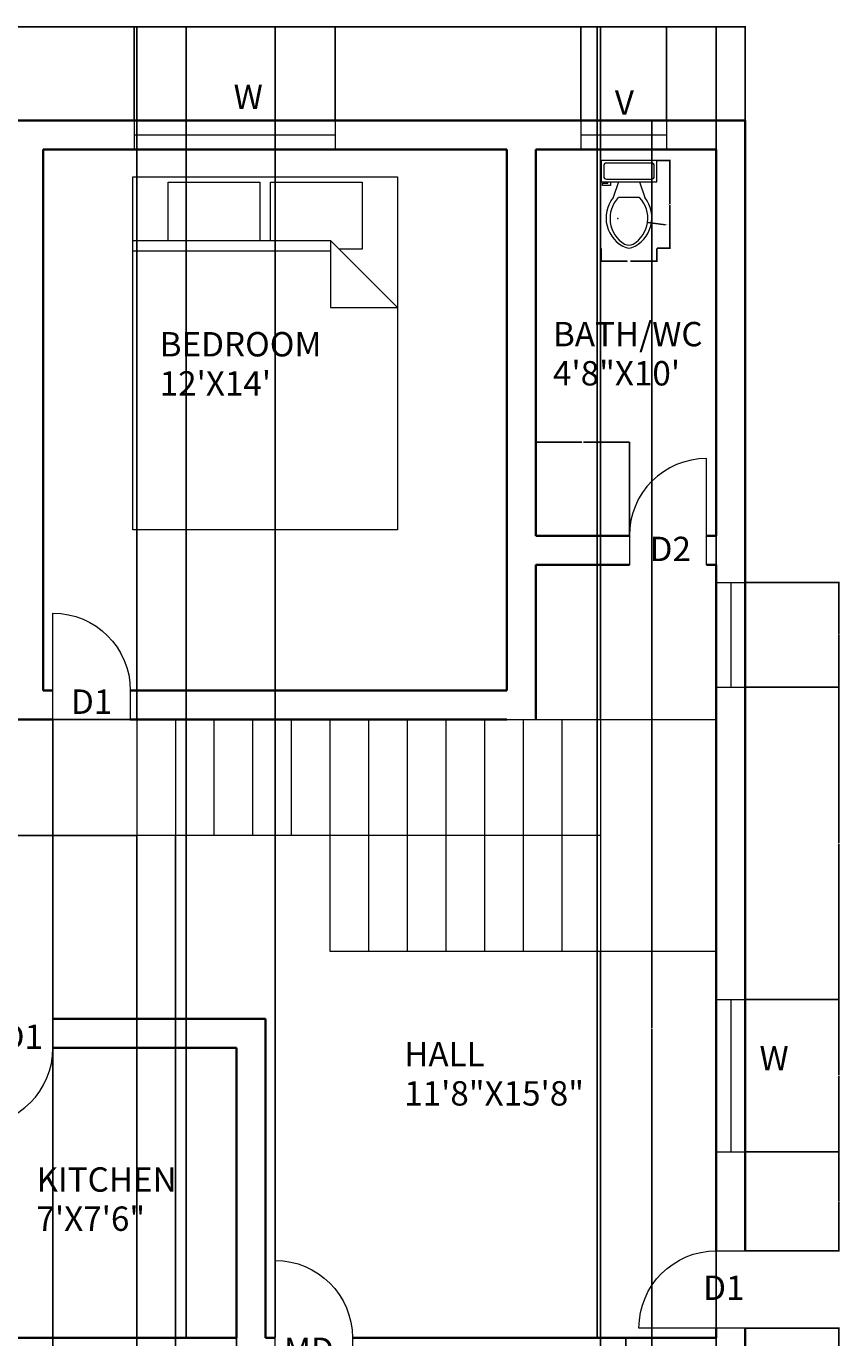
# Model space of a CAD drawing. Units: feet. Extents: x 2075 to 2525, y 1791 to 2414.
# Tile 3 of 3: x 2273 to 2525, y 2006 to 2414. Entities that reach past the tile are written whole.
import ezdxf

# ---------------------------------------------------------------- set-up
doc = ezdxf.new("R2010")
doc.units = ezdxf.units.FT
for name, color, linetype, lineweight in [('A-ANNO-DIMS', 2, 'Continuous', 18), ('A-ANNO-TEXT', 7, 'Continuous', 18), ('A-AREA-IDEN', 7, 'Continuous', 18), ('A-DOOR', 3, 'Continuous', 18), ('A-FLOR-FIXT', 8, 'Continuous', 18), ('A-FLOR-STRS', 7, 'Continuous', 18), ('A-FURN', 8, 'Continuous', 18), ('A-GLAZ', 4, 'Continuous', 18), ('A-WALL', 7, 'Continuous', 35)]:
    doc.layers.add(name, color=color, linetype=linetype, lineweight=lineweight)
doc.styles.get("Standard").update_dxf_attribs({"font": 'arial.ttf'})
doc.dimstyles.get("Standard").update_dxf_attribs({"dimtxt": 0.18, "dimasz": 0.18, "dimexe": 0.18, "dimexo": 0.0625, "dimgap": 0.09, "dimtad": 0, "dimtih": 1, "dimtoh": 1, "dimdec": 4, "dimzin": 0, "dimdsep": 46, "dimtxsty": 'Standard', "dimcen": 0.09, "dimadec": 0, "dimazin": 0, "dimtfac": 1, "dimtdec": 4, "dimtofl": 0, "dimtmove": 0, "dimatfit": 3, "dimfxl": 1, "dimtolj": 1, "dimtzin": 0, "dimarcsym": 0})

# ---------------------------------------------------------------- blocks, each defined once
blk = doc.blocks.new('Toilet - top')
for p, q in [((9.5, -6), (9.5, -2)), ((-10, -8.5), (-8, -8.5)), ((-10, -9.5), (-10, -8.5)), ((-7, -9.5), (-10, -9.5)), ((-8, -8.5), (-8, -8)), ((-7, -8), (-7, -9.5)), ((-4, -8), (-6, -14)), ((4, -8), (6, -14)), ((4, -14), (-4, -14))]:
    blk.add_line(p, q)
blk.add_lwpolyline([(10.5, -8), (10.5, 0), (-10.5, 0), (-10.5, -8)], close=True)
for points in [[(-9.5, -2), (-9.5, -6)], [(8.5, -1), (-8.5, -1)], [(-8.5, -7), (8.5, -7)]]:
    blk.add_lwpolyline(points)
for centre, radius, start, end in [((-8.62, -1.88), 0.884, 81.8699, 188.1301), ((8.62, -1.88), 0.884, 351.8699, 98.1301), ((-8.62, -6.12), 0.884, 171.8699, 278.1301), ((8.62, -6.12), 0.884, 261.8699, 8.1301), ((3.52, -21.58), 12.17, 141.4691, 247.9714), ((4.2, -21.82), 11.33, 136.3677, 238.9468), ((-3.52, -21.58), 12.17, 292.0284, 38.5307), ((-4.2, -21.82), 11.33, 301.053, 43.6321), ((0, -27.88), 4, 245.7318, 294.2682), ((0, -29), 4, 254.8605, 285.1395)]:
    blk.add_arc(centre, radius, start, end)
blk = doc.blocks.new('Bed - Queen')
for p, q in [((0, -80.00003), (0, 0)), ((0, 0), (59.99999, 0)), ((59.99999, 0), (59.99999, -80.00003)), ((7.99999, -1.2), (28.79998, -1.2)), ((7.99999, -14.4), (7.99999, -1.2)), ((28.79998, -1.2), (28.79998, -14.4)), ((31.19999, -1.2), (51.99999, -1.2)), ((31.19999, -14.4), (31.19999, -1.2)), ((51.99999, -1.2), (51.99999, -16.4)), ((0, -14.4), (44.8, -14.4)), ((59.99999, -29.6), (44.8, -14.4)), ((44.8, -14.4), (44.8, -29.6)), ((44.8, -16.8), (0, -16.8)), ((51.99999, -16.4), (46.79936, -16.4)), ((44.8, -29.6), (59.99999, -29.6)), ((59.99999, -80.00003), (0, -80.00003))]:
    blk.add_line(p, q)
blk = doc.blocks.new('DOOR-SINGLE-SWING')
for p, q in [((24, 0), (24, 33)), ((0, 9), (0, 0))]:
    blk.add_line(p, q)
blk.add_arc((24, 9), 24, 90, 180)
blk = doc.blocks.new('*D9')
at = {"layer": 'A-ANNO-DIMS', "color": 0, "lineweight": -2, "transparency": 16777216}
for p, q in [((2468.52, 2371.88), (2472.72, 2371.88)), ((2472.54, 2371.7), (2472.54, 2358.45)), ((2472.54, 2344.84), (2472.54, 2358.09)), ((2468.52, 2344.66), (2472.72, 2344.66))]:
    blk.add_line(p, q, dxfattribs=at)
at = {"layer": 'A-ANNO-DIMS', "color": 0, "transparency": 16777216}
for points in [[(2472.51, 2371.7), (2472.57, 2371.7), (2472.54, 2371.88)], [(2472.51, 2344.84), (2472.57, 2344.84), (2472.54, 2344.66)]]:
    blk.add_solid(points, dxfattribs=at)
at = {"layer": 'Defpoints', "color": 0, "transparency": 16777216}
for p in [(2468.46, 2371.88), (2472.54, 2371.88), (2468.46, 2344.66)]:
    blk.add_point(p, dxfattribs=at)
at = {"layer": 'A-ANNO-DIMS', "color": 0, "transparency": 16777216, "insert": (2472.54, 2358.27), "char_height": 0.18, "attachment_point": 5}
blk.add_mtext('\\A1;WC 27 TYP.', dxfattribs=at)
blk = doc.blocks.new('*D10')
at = {"layer": 'A-ANNO-DIMS', "color": 0, "lineweight": -2, "transparency": 16777216}
for p, q in [((2451.16, 2344.59), (2451.16, 2340.39)), ((2468.46, 2344.59), (2468.46, 2340.39)), ((2451.34, 2340.57), (2459.29, 2340.57)), ((2468.28, 2340.57), (2460.33, 2340.57))]:
    blk.add_line(p, q, dxfattribs=at)
at = {"layer": 'A-ANNO-DIMS', "color": 0, "transparency": 16777216}
for points in [[(2451.34, 2340.6), (2451.34, 2340.54), (2451.16, 2340.57)], [(2468.28, 2340.6), (2468.28, 2340.54), (2468.46, 2340.57)]]:
    blk.add_solid(points, dxfattribs=at)
at = {"layer": 'Defpoints', "color": 0, "transparency": 16777216}
for p in [(2451.16, 2344.66), (2468.46, 2344.66), (2468.46, 2340.57)]:
    blk.add_point(p, dxfattribs=at)
at = {"layer": 'A-ANNO-DIMS', "color": 0, "transparency": 16777216, "insert": (2459.81, 2340.57), "char_height": 0.18, "attachment_point": 5}
blk.add_mtext('\\A1;17 TYP.', dxfattribs=at)
blk = doc.blocks.new('*D12')
at = {"layer": 'A-ANNO-DIMS', "color": 0, "lineweight": -2, "transparency": 16777216}
for p, q in [((2449.99, 2006.33), (2458.98, 2006.33)), ((2458.8, 2006.15), (2458.8, 2002.01)), ((2458.8, 1997.51), (2458.8, 2001.65)), ((2449.99, 1997.33), (2458.98, 1997.33))]:
    blk.add_line(p, q, dxfattribs=at)
at = {"layer": 'A-ANNO-DIMS', "color": 0, "transparency": 16777216}
for points in [[(2458.77, 2006.15), (2458.83, 2006.15), (2458.8, 2006.33)], [(2458.77, 1997.51), (2458.83, 1997.51), (2458.8, 1997.33)]]:
    blk.add_solid(points, dxfattribs=at)
at = {"layer": 'Defpoints', "color": 0, "transparency": 16777216}
for p in [(2449.92, 2006.33), (2458.8, 2006.33), (2449.92, 1997.33)]:
    blk.add_point(p, dxfattribs=at)
at = {"layer": 'A-ANNO-DIMS', "color": 0, "transparency": 16777216, "insert": (2458.8, 2001.83), "char_height": 0.18, "attachment_point": 5}
blk.add_mtext('\\A1;9 TYP.', dxfattribs=at)
blk = doc.blocks.new('*D14')
at = {"layer": 'A-ANNO-DIMS', "color": 0, "lineweight": -2, "transparency": 16777216}
for p, q in [((2495.87, 2384.33), (2466.7, 2384.33)), ((2466.88, 2384.15), (2466.88, 2102.51)), ((2466.88, 1820.51), (2466.88, 2102.15)), ((2495.87, 1820.33), (2466.7, 1820.33))]:
    blk.add_line(p, q, dxfattribs=at)
at = {"layer": 'A-ANNO-DIMS', "color": 0, "transparency": 16777216}
for points in [[(2466.85, 2384.15), (2466.91, 2384.15), (2466.88, 2384.33)], [(2466.85, 1820.51), (2466.91, 1820.51), (2466.88, 1820.33)]]:
    blk.add_solid(points, dxfattribs=at)
at = {"layer": 'Defpoints', "color": 0, "transparency": 16777216}
for p in [(2466.88, 2384.33), (2495.93, 2384.33), (2495.93, 1820.33)]:
    blk.add_point(p, dxfattribs=at)
at = {"layer": 'A-ANNO-DIMS', "color": 0, "transparency": 16777216, "insert": (2466.88, 2102.33), "char_height": 0.18, "attachment_point": 5}
blk.add_mtext('\\A1;564', dxfattribs=at)
blk = doc.blocks.new('*D17')
at = {"layer": 'A-ANNO-DIMS', "color": 0, "lineweight": -2, "transparency": 16777216}
for p, q in [((2306.93, 2198.39), (2306.93, 2413.56)), ((2307.11, 2413.38), (2378.65, 2413.38)), ((2450.75, 2413.38), (2379.21, 2413.38)), ((2450.93, 2198.39), (2450.93, 2413.56))]:
    blk.add_line(p, q, dxfattribs=at)
at = {"layer": 'A-ANNO-DIMS', "color": 0, "transparency": 16777216}
for points in [[(2307.11, 2413.41), (2307.11, 2413.35), (2306.93, 2413.38)], [(2450.75, 2413.41), (2450.75, 2413.35), (2450.93, 2413.38)]]:
    blk.add_solid(points, dxfattribs=at)
at = {"layer": 'Defpoints', "color": 0, "transparency": 16777216}
for p in [(2450.93, 2413.38), (2306.93, 2198.33), (2450.93, 2198.33)]:
    blk.add_point(p, dxfattribs=at)
at = {"layer": 'A-ANNO-DIMS', "color": 0, "transparency": 16777216, "insert": (2378.93, 2413.38), "char_height": 0.18, "attachment_point": 5}
blk.add_mtext('\\A1;144', dxfattribs=at)
blk = doc.blocks.new('*D18')
at = {"layer": 'A-ANNO-DIMS', "color": 0, "lineweight": -2, "transparency": 16777216}
for p, q in [((2450.93, 2126.27), (2450.93, 1791.1)), ((2486.93, 2126.27), (2486.93, 1791.1)), ((2451.11, 1791.28), (2468.71, 1791.28)), ((2486.75, 1791.28), (2469.15, 1791.28))]:
    blk.add_line(p, q, dxfattribs=at)
at = {"layer": 'A-ANNO-DIMS', "color": 0, "transparency": 16777216}
for points in [[(2451.11, 1791.31), (2451.11, 1791.25), (2450.93, 1791.28)], [(2486.75, 1791.31), (2486.75, 1791.25), (2486.93, 1791.28)]]:
    blk.add_solid(points, dxfattribs=at)
at = {"layer": 'Defpoints', "color": 0, "transparency": 16777216}
for p in [(2450.93, 2126.33), (2486.93, 2126.33), (2486.93, 1791.28)]:
    blk.add_point(p, dxfattribs=at)
at = {"layer": 'A-ANNO-DIMS', "color": 0, "transparency": 16777216, "insert": (2468.93, 1791.28), "char_height": 0.18, "attachment_point": 5}
blk.add_mtext('\\A1;36', dxfattribs=at)
blk = doc.blocks.new('*D19')
at = {"layer": 'A-ANNO-DIMS', "color": 0, "lineweight": -2, "transparency": 16777216}
for p, q in [((2306.87, 2198.33), (2074.7, 2198.33)), ((2074.88, 2198.15), (2074.88, 2180.51)), ((2074.88, 2162.51), (2074.88, 2180.15)), ((2306.87, 2162.33), (2074.7, 2162.33))]:
    blk.add_line(p, q, dxfattribs=at)
at = {"layer": 'A-ANNO-DIMS', "color": 0, "transparency": 16777216}
for points in [[(2074.85, 2198.15), (2074.91, 2198.15), (2074.88, 2198.33)], [(2074.85, 2162.51), (2074.91, 2162.51), (2074.88, 2162.33)]]:
    blk.add_solid(points, dxfattribs=at)
at = {"layer": 'Defpoints', "color": 0, "transparency": 16777216}
for p in [(2074.88, 2198.33), (2306.93, 2198.33), (2306.93, 2162.33)]:
    blk.add_point(p, dxfattribs=at)
at = {"layer": 'A-ANNO-DIMS', "color": 0, "transparency": 16777216, "insert": (2074.88, 2180.33), "char_height": 0.18, "attachment_point": 5}
blk.add_mtext('\\A1;36', dxfattribs=at)
blk = doc.blocks.new('*D20')
at = {"layer": 'A-ANNO-DIMS', "color": 0, "lineweight": -2, "transparency": 16777216}
for p, q in [((2306.93, 2162.27), (2306.93, 1791.1)), ((2318.93, 2162.27), (2318.93, 1791.1)), ((2307.11, 1791.28), (2312.72, 1791.28)), ((2318.75, 1791.28), (2313.14, 1791.28))]:
    blk.add_line(p, q, dxfattribs=at)
at = {"layer": 'A-ANNO-DIMS', "color": 0, "transparency": 16777216}
for points in [[(2307.11, 1791.31), (2307.11, 1791.25), (2306.93, 1791.28)], [(2318.75, 1791.31), (2318.75, 1791.25), (2318.93, 1791.28)]]:
    blk.add_solid(points, dxfattribs=at)
at = {"layer": 'Defpoints', "color": 0, "transparency": 16777216}
for p in [(2306.93, 2162.33), (2318.93, 2162.33), (2318.93, 1791.28)]:
    blk.add_point(p, dxfattribs=at)
at = {"layer": 'A-ANNO-DIMS', "color": 0, "transparency": 16777216, "insert": (2312.93, 1791.28), "char_height": 0.18, "attachment_point": 5}
blk.add_mtext('\\A1;12', dxfattribs=at)
blk = doc.blocks.new('*D23')
at = {"layer": 'A-ANNO-DIMS', "color": 0, "lineweight": -2, "transparency": 16777216}
for p, q in [((2209.78, 2384.39), (2209.78, 2413.56)), ((2209.96, 2413.38), (2257.59, 2413.38)), ((2306.01, 2413.38), (2258.38, 2413.38)), ((2306.19, 2384.39), (2306.19, 2413.56))]:
    blk.add_line(p, q, dxfattribs=at)
at = {"layer": 'A-ANNO-DIMS', "color": 0, "transparency": 16777216}
for points in [[(2209.96, 2413.41), (2209.96, 2413.35), (2209.78, 2413.38)], [(2306.01, 2413.41), (2306.01, 2413.35), (2306.19, 2413.38)]]:
    blk.add_solid(points, dxfattribs=at)
at = {"layer": 'Defpoints', "color": 0, "transparency": 16777216}
for p in [(2306.19, 2413.38), (2209.78, 2384.33), (2306.19, 2384.33)]:
    blk.add_point(p, dxfattribs=at)
at = {"layer": 'A-ANNO-DIMS', "color": 0, "transparency": 16777216, "insert": (2257.98, 2413.38), "char_height": 0.18, "attachment_point": 5}
blk.add_mtext('\\A1;96.42', dxfattribs=at)
blk = doc.blocks.new('*D24')
at = {"layer": 'A-ANNO-DIMS', "color": 0, "lineweight": -2, "transparency": 16777216}
for p, q in [((2306.19, 2384.39), (2306.19, 2413.56)), ((2306.37, 2413.38), (2336.97, 2413.38)), ((2368.36, 2413.38), (2337.76, 2413.38)), ((2368.54, 2384.39), (2368.54, 2413.56))]:
    blk.add_line(p, q, dxfattribs=at)
at = {"layer": 'A-ANNO-DIMS', "color": 0, "transparency": 16777216}
for points in [[(2306.37, 2413.41), (2306.37, 2413.35), (2306.19, 2413.38)], [(2368.36, 2413.41), (2368.36, 2413.35), (2368.54, 2413.38)]]:
    blk.add_solid(points, dxfattribs=at)
at = {"layer": 'Defpoints', "color": 0, "transparency": 16777216}
for p in [(2368.54, 2413.38), (2306.19, 2384.33), (2368.54, 2384.33)]:
    blk.add_point(p, dxfattribs=at)
at = {"layer": 'A-ANNO-DIMS', "color": 0, "transparency": 16777216, "insert": (2337.37, 2413.38), "char_height": 0.18, "attachment_point": 5}
blk.add_mtext('\\A1;62.35', dxfattribs=at)
blk = doc.blocks.new('*D25')
at = {"layer": 'A-ANNO-DIMS', "color": 0, "lineweight": -2, "transparency": 16777216}
for p, q in [((2368.54, 2384.39), (2368.54, 2413.56)), ((2368.72, 2413.38), (2406.32, 2413.38)), ((2444.7, 2413.38), (2407.1, 2413.38)), ((2444.88, 2384.39), (2444.88, 2413.56))]:
    blk.add_line(p, q, dxfattribs=at)
at = {"layer": 'A-ANNO-DIMS', "color": 0, "transparency": 16777216}
for points in [[(2368.72, 2413.41), (2368.72, 2413.35), (2368.54, 2413.38)], [(2444.7, 2413.41), (2444.7, 2413.35), (2444.88, 2413.38)]]:
    blk.add_solid(points, dxfattribs=at)
at = {"layer": 'Defpoints', "color": 0, "transparency": 16777216}
for p in [(2444.88, 2413.38), (2368.54, 2384.33), (2444.88, 2384.33)]:
    blk.add_point(p, dxfattribs=at)
at = {"layer": 'A-ANNO-DIMS', "color": 0, "transparency": 16777216, "insert": (2406.71, 2413.38), "char_height": 0.18, "attachment_point": 5}
blk.add_mtext('\\A1;76.33', dxfattribs=at)
blk = doc.blocks.new('*D26')
at = {"layer": 'A-ANNO-DIMS', "color": 0, "lineweight": -2, "transparency": 16777216}
for p, q in [((2444.88, 2384.39), (2444.88, 2413.56)), ((2445.06, 2413.38), (2457.68, 2413.38)), ((2471.24, 2413.38), (2458.61, 2413.38)), ((2471.42, 2384.39), (2471.42, 2413.56))]:
    blk.add_line(p, q, dxfattribs=at)
at = {"layer": 'A-ANNO-DIMS', "color": 0, "transparency": 16777216}
for points in [[(2445.06, 2413.41), (2445.06, 2413.35), (2444.88, 2413.38)], [(2471.24, 2413.41), (2471.24, 2413.35), (2471.42, 2413.38)]]:
    blk.add_solid(points, dxfattribs=at)
at = {"layer": 'Defpoints', "color": 0, "transparency": 16777216}
for p in [(2471.42, 2413.38), (2444.88, 2384.33), (2471.42, 2384.33)]:
    blk.add_point(p, dxfattribs=at)
at = {"layer": 'A-ANNO-DIMS', "color": 0, "transparency": 16777216, "insert": (2458.15, 2413.38), "char_height": 0.18, "attachment_point": 5}
blk.add_mtext('\\A1;26.543', dxfattribs=at)
blk = doc.blocks.new('*D27')
at = {"layer": 'A-ANNO-DIMS', "color": 0, "lineweight": -2, "transparency": 16777216}
for p, q in [((2471.42, 2384.39), (2471.42, 2413.56)), ((2471.6, 2413.38), (2483.3, 2413.38)), ((2495.75, 2413.38), (2484.05, 2413.38)), ((2495.93, 2384.39), (2495.93, 2413.56))]:
    blk.add_line(p, q, dxfattribs=at)
at = {"layer": 'A-ANNO-DIMS', "color": 0, "transparency": 16777216}
for points in [[(2471.6, 2413.41), (2471.6, 2413.35), (2471.42, 2413.38)], [(2495.75, 2413.41), (2495.75, 2413.35), (2495.93, 2413.38)]]:
    blk.add_solid(points, dxfattribs=at)
at = {"layer": 'Defpoints', "color": 0, "transparency": 16777216}
for p in [(2495.93, 2413.38), (2471.42, 2384.33), (2495.93, 2384.33)]:
    blk.add_point(p, dxfattribs=at)
at = {"layer": 'A-ANNO-DIMS', "color": 0, "transparency": 16777216, "insert": (2483.67, 2413.38), "char_height": 0.18, "attachment_point": 5}
blk.add_mtext('\\A1;24.51', dxfattribs=at)
blk = doc.blocks.new('*D37')
at = {"layer": 'A-ANNO-DIMS', "color": 0, "lineweight": -2, "transparency": 16777216}
for p, q in [((2495.99, 2009.33), (2525.16, 2009.33)), ((2524.98, 2009.15), (2524.98, 2003.51)), ((2524.98, 1997.51), (2524.98, 2003.15)), ((2495.99, 1997.33), (2525.16, 1997.33))]:
    blk.add_line(p, q, dxfattribs=at)
at = {"layer": 'A-ANNO-DIMS', "color": 0, "transparency": 16777216}
for points in [[(2524.95, 2009.15), (2525.01, 2009.15), (2524.98, 2009.33)], [(2524.95, 1997.51), (2525.01, 1997.51), (2524.98, 1997.33)]]:
    blk.add_solid(points, dxfattribs=at)
at = {"layer": 'Defpoints', "color": 0, "transparency": 16777216}
for p in [(2495.93, 2009.33), (2524.98, 2009.33), (2495.93, 1997.33)]:
    blk.add_point(p, dxfattribs=at)
at = {"layer": 'A-ANNO-DIMS', "color": 0, "transparency": 16777216, "insert": (2524.98, 2003.33), "char_height": 0.18, "attachment_point": 5}
blk.add_mtext('\\A1;12', dxfattribs=at)
blk = doc.blocks.new('*D38')
at = {"layer": 'A-ANNO-DIMS', "color": 0, "lineweight": -2, "transparency": 16777216}
for p, q in [((2495.99, 2064.11), (2525.16, 2064.11)), ((2524.98, 2063.93), (2524.98, 2048.9)), ((2524.98, 2033.51), (2524.98, 2048.54)), ((2495.99, 2033.33), (2525.16, 2033.33))]:
    blk.add_line(p, q, dxfattribs=at)
at = {"layer": 'A-ANNO-DIMS', "color": 0, "transparency": 16777216}
for points in [[(2524.95, 2063.93), (2525.01, 2063.93), (2524.98, 2064.11)], [(2524.95, 2033.51), (2525.01, 2033.51), (2524.98, 2033.33)]]:
    blk.add_solid(points, dxfattribs=at)
at = {"layer": 'Defpoints', "color": 0, "transparency": 16777216}
for p in [(2495.93, 2064.11), (2524.98, 2064.11), (2495.93, 2033.33)]:
    blk.add_point(p, dxfattribs=at)
at = {"layer": 'A-ANNO-DIMS', "color": 0, "transparency": 16777216, "insert": (2524.98, 2048.72), "char_height": 0.18, "attachment_point": 5}
blk.add_mtext('\\A1;30.78', dxfattribs=at)
blk = doc.blocks.new('*D39')
at = {"layer": 'A-ANNO-DIMS', "color": 0, "lineweight": -2, "transparency": 16777216}
for p, q in [((2495.99, 2111.33), (2525.16, 2111.33)), ((2524.98, 2111.15), (2524.98, 2087.9)), ((2524.98, 2064.29), (2524.98, 2087.54)), ((2495.99, 2064.11), (2525.16, 2064.11))]:
    blk.add_line(p, q, dxfattribs=at)
at = {"layer": 'A-ANNO-DIMS', "color": 0, "transparency": 16777216}
for points in [[(2524.95, 2111.15), (2525.01, 2111.15), (2524.98, 2111.33)], [(2524.95, 2064.29), (2525.01, 2064.29), (2524.98, 2064.11)]]:
    blk.add_solid(points, dxfattribs=at)
at = {"layer": 'Defpoints', "color": 0, "transparency": 16777216}
for p in [(2495.93, 2111.33), (2524.98, 2111.33), (2495.93, 2064.11)]:
    blk.add_point(p, dxfattribs=at)
at = {"layer": 'A-ANNO-DIMS', "color": 0, "transparency": 16777216, "insert": (2524.98, 2087.72), "char_height": 0.18, "attachment_point": 5}
blk.add_mtext('\\A1;47.22', dxfattribs=at)
blk = doc.blocks.new('*D40')
at = {"layer": 'A-ANNO-DIMS', "color": 0, "lineweight": -2, "transparency": 16777216}
for p, q in [((2495.99, 2208.39), (2525.16, 2208.39)), ((2524.98, 2208.21), (2524.98, 2160.04)), ((2524.98, 2111.51), (2524.98, 2159.68)), ((2495.99, 2111.33), (2525.16, 2111.33))]:
    blk.add_line(p, q, dxfattribs=at)
at = {"layer": 'A-ANNO-DIMS', "color": 0, "transparency": 16777216}
for points in [[(2524.95, 2208.21), (2525.01, 2208.21), (2524.98, 2208.39)], [(2524.95, 2111.51), (2525.01, 2111.51), (2524.98, 2111.33)]]:
    blk.add_solid(points, dxfattribs=at)
at = {"layer": 'Defpoints', "color": 0, "transparency": 16777216}
for p in [(2495.93, 2208.39), (2524.98, 2208.39), (2495.93, 2111.33)]:
    blk.add_point(p, dxfattribs=at)
at = {"layer": 'A-ANNO-DIMS', "color": 0, "transparency": 16777216, "insert": (2524.98, 2159.86), "char_height": 0.18, "attachment_point": 5}
blk.add_mtext('\\A1;97.06', dxfattribs=at)
blk = doc.blocks.new('*D41')
at = {"layer": 'A-ANNO-DIMS', "color": 0, "lineweight": -2, "transparency": 16777216}
for p, q in [((2495.99, 2240.85), (2525.16, 2240.85)), ((2524.98, 2240.67), (2524.98, 2224.8)), ((2524.98, 2208.57), (2524.98, 2224.44)), ((2495.99, 2208.39), (2525.16, 2208.39))]:
    blk.add_line(p, q, dxfattribs=at)
at = {"layer": 'A-ANNO-DIMS', "color": 0, "transparency": 16777216}
for points in [[(2524.95, 2240.67), (2525.01, 2240.67), (2524.98, 2240.85)], [(2524.95, 2208.57), (2525.01, 2208.57), (2524.98, 2208.39)]]:
    blk.add_solid(points, dxfattribs=at)
at = {"layer": 'Defpoints', "color": 0, "transparency": 16777216}
for p in [(2495.93, 2240.85), (2524.98, 2240.85), (2495.93, 2208.39)]:
    blk.add_point(p, dxfattribs=at)
at = {"layer": 'A-ANNO-DIMS', "color": 0, "transparency": 16777216, "insert": (2524.98, 2224.62), "char_height": 0.18, "attachment_point": 5}
blk.add_mtext('\\A1;32.46', dxfattribs=at)
blk = doc.blocks.new('*D45')
at = {"layer": 'A-ANNO-DIMS', "color": 0, "lineweight": -2, "transparency": 16777216}
for p, q in [((2322.27, 2006.39), (2322.27, 2413.56)), ((2322.45, 2413.38), (2335.7, 2413.38)), ((2349.75, 2413.38), (2336.49, 2413.38)), ((2349.93, 2006.39), (2349.93, 2413.56))]:
    blk.add_line(p, q, dxfattribs=at)
at = {"layer": 'A-ANNO-DIMS', "color": 0, "transparency": 16777216}
for points in [[(2322.45, 2413.41), (2322.45, 2413.35), (2322.27, 2413.38)], [(2349.75, 2413.41), (2349.75, 2413.35), (2349.93, 2413.38)]]:
    blk.add_solid(points, dxfattribs=at)
at = {"layer": 'Defpoints', "color": 0, "transparency": 16777216}
for p in [(2349.93, 2413.38), (2322.27, 2006.33), (2349.93, 2006.33)]:
    blk.add_point(p, dxfattribs=at)
at = {"layer": 'A-ANNO-DIMS', "color": 0, "transparency": 16777216, "insert": (2336.1, 2413.38), "char_height": 0.18, "attachment_point": 5}
blk.add_mtext('\\A1;27.66', dxfattribs=at)
blk = doc.blocks.new('*D47')
at = {"layer": 'A-ANNO-DIMS', "color": 0, "lineweight": -2, "transparency": 16777216}
for p, q in [((2449.92, 2006.39), (2449.92, 2413.56)), ((2450.1, 2413.38), (2468.21, 2413.38)), ((2486.75, 2413.38), (2468.65, 2413.38)), ((2486.93, 2006.39), (2486.93, 2413.56))]:
    blk.add_line(p, q, dxfattribs=at)
at = {"layer": 'A-ANNO-DIMS', "color": 0, "transparency": 16777216}
for points in [[(2450.1, 2413.41), (2450.1, 2413.35), (2449.92, 2413.38)], [(2486.75, 2413.41), (2486.75, 2413.35), (2486.93, 2413.38)]]:
    blk.add_solid(points, dxfattribs=at)
at = {"layer": 'Defpoints', "color": 0, "transparency": 16777216}
for p in [(2486.93, 2413.38), (2449.92, 2006.33), (2486.93, 2006.33)]:
    blk.add_point(p, dxfattribs=at)
at = {"layer": 'A-ANNO-DIMS', "color": 0, "transparency": 16777216, "insert": (2468.43, 2413.38), "char_height": 0.18, "attachment_point": 5}
blk.add_mtext('\\A1;37', dxfattribs=at)
blk = doc.blocks.new('*D48')
at = {"layer": 'A-ANNO-DIMS', "color": 0, "lineweight": -2, "transparency": 16777216}
for p, q in [((2265.93, 2198.27), (2265.93, 1791.1)), ((2280.93, 2198.27), (2280.93, 1791.1)), ((2266.11, 1791.28), (2273.22, 1791.28)), ((2280.75, 1791.28), (2273.64, 1791.28))]:
    blk.add_line(p, q, dxfattribs=at)
at = {"layer": 'A-ANNO-DIMS', "color": 0, "transparency": 16777216}
for points in [[(2266.11, 1791.31), (2266.11, 1791.25), (2265.93, 1791.28)], [(2280.75, 1791.31), (2280.75, 1791.25), (2280.93, 1791.28)]]:
    blk.add_solid(points, dxfattribs=at)
at = {"layer": 'Defpoints', "color": 0, "transparency": 16777216}
for p in [(2265.93, 2198.33), (2280.93, 2198.33), (2280.93, 1791.28)]:
    blk.add_point(p, dxfattribs=at)
at = {"layer": 'A-ANNO-DIMS', "color": 0, "transparency": 16777216, "insert": (2273.43, 1791.28), "char_height": 0.18, "attachment_point": 5}
blk.add_mtext('\\A1;15', dxfattribs=at)
blk = doc.blocks.new('*D49')
at = {"layer": 'A-ANNO-DIMS', "color": 0, "lineweight": -2, "transparency": 16777216}
for p, q in [((2430.93, 2255.39), (2430.93, 2284.56)), ((2459.93, 2255.39), (2459.93, 2284.56)), ((2431.11, 2284.38), (2445.21, 2284.38)), ((2459.75, 2284.38), (2445.65, 2284.38))]:
    blk.add_line(p, q, dxfattribs=at)
at = {"layer": 'A-ANNO-DIMS', "color": 0, "transparency": 16777216}
for points in [[(2431.11, 2284.41), (2431.11, 2284.35), (2430.93, 2284.38)], [(2459.75, 2284.41), (2459.75, 2284.35), (2459.93, 2284.38)]]:
    blk.add_solid(points, dxfattribs=at)
at = {"layer": 'Defpoints', "color": 0, "transparency": 16777216}
for p in [(2459.93, 2284.38), (2430.93, 2255.33), (2459.93, 2255.33)]:
    blk.add_point(p, dxfattribs=at)
at = {"layer": 'A-ANNO-DIMS', "color": 0, "transparency": 16777216, "insert": (2445.43, 2284.38), "char_height": 0.18, "attachment_point": 5}
blk.add_mtext('\\A1;29', dxfattribs=at)
blk = doc.blocks.new('*D51')
at = {"layer": 'A-ANNO-DIMS', "color": 0, "lineweight": -2, "transparency": 16777216}
for p, q in [((2280.93, 2096.27), (2280.93, 1791.1)), ((2337.93, 2096.27), (2337.93, 1791.1)), ((2281.11, 1791.28), (2309.21, 1791.28)), ((2337.75, 1791.28), (2309.65, 1791.28))]:
    blk.add_line(p, q, dxfattribs=at)
at = {"layer": 'A-ANNO-DIMS', "color": 0, "transparency": 16777216}
for points in [[(2281.11, 1791.31), (2281.11, 1791.25), (2280.93, 1791.28)], [(2337.75, 1791.31), (2337.75, 1791.25), (2337.93, 1791.28)]]:
    blk.add_solid(points, dxfattribs=at)
at = {"layer": 'Defpoints', "color": 0, "transparency": 16777216}
for p in [(2280.93, 2096.33), (2337.93, 2096.33), (2337.93, 1791.28)]:
    blk.add_point(p, dxfattribs=at)
at = {"layer": 'A-ANNO-DIMS', "color": 0, "transparency": 16777216, "insert": (2309.43, 1791.28), "char_height": 0.18, "attachment_point": 5}
blk.add_mtext('\\A1;57', dxfattribs=at)
blk = doc.blocks.new('*D56')
at = {"layer": 'A-ANNO-DIMS', "color": 0, "lineweight": -2, "transparency": 16777216}
for p, q in [((2456.26, 2353.91), (2456.44, 2353.91)), ((2456.35, 2353.82), (2456.35, 2354)), ((2471.15, 2351.92), (2465.78, 2352.64))]:
    blk.add_line(p, q, dxfattribs=at)
at = {"layer": 'A-ANNO-DIMS', "color": 0, "transparency": 16777216}
blk.add_solid([(2465.78, 2352.67), (2465.77, 2352.61), (2465.6, 2352.67)], dxfattribs=at)
at = {"layer": 'Defpoints', "color": 0, "transparency": 16777216}
for p in [(2456.35, 2353.91), (2465.6, 2352.67)]:
    blk.add_point(p, dxfattribs=at)
at = {"layer": 'A-ANNO-DIMS', "color": 0, "transparency": 16777216, "insert": (2471.83, 2351.92), "char_height": 0.18, "attachment_point": 5}
blk.add_mtext('\\A1;4X R9.335', dxfattribs=at)

msp = doc.modelspace()

# ---------------------------------------------------------------- linework, layer by layer
at = {"layer": 'A-FLOR-STRS'}
for p, q in [((2304.9279, 2198.3311), (2486.9279, 2198.3311)), ((2306.9279, 2198.3311), (2306.9279, 2162.3311)), ((2318.9279, 2198.3311), (2318.9279, 2162.3311)), ((2330.9279, 2198.3311), (2330.9279, 2162.3311)), ((2342.9279, 2198.3311), (2342.9279, 2162.3311)), ((2354.9279, 2198.3311), (2354.9279, 2162.3311)), ((2366.9279, 2198.3311), (2366.9279, 2126.3311)), ((2378.9279, 2198.3311), (2378.9279, 2126.3311)), ((2390.9279, 2198.3311), (2390.9279, 2126.3311)), ((2402.9279, 2198.3311), (2402.9279, 2126.3311)), ((2414.9279, 2198.3311), (2414.9279, 2126.3311)), ((2426.9279, 2198.3311), (2426.9279, 2126.3311)), ((2438.9279, 2198.3311), (2438.9279, 2126.3311)), ((2450.9279, 2198.3311), (2450.9279, 2126.3311)), ((2450.9279, 2162.3311), (2306.9279, 2162.3311)), ((2366.9279, 2126.3311), (2486.9279, 2126.3311))]:
    msp.add_line(p, q, dxfattribs=at)
at = {"layer": 'A-GLAZ'}
for p, q in [((2306.1931, 2384.3311), (2306.1931, 2375.3311)), ((2368.544, 2384.3311), (2368.544, 2375.3311)), ((2444.8768, 2384.3311), (2444.8768, 2375.3311)), ((2471.4201, 2384.3311), (2471.4201, 2375.3311)), ((2306.1931, 2379.8311), (2368.544, 2379.8311)), ((2444.8768, 2379.8311), (2471.4201, 2379.8311)), ((2486.9279, 2240.8536), (2495.9279, 2240.8536)), ((2491.4279, 2240.8536), (2491.4279, 2208.3905)), ((2486.9279, 2208.3905), (2495.9279, 2208.3905)), ((2486.9279, 2111.3282), (2495.9279, 2111.3282)), ((2491.4279, 2111.3282), (2491.4279, 2064.1084)), ((2486.9279, 2064.1084), (2495.9279, 2064.1084))]:
    msp.add_line(p, q, dxfattribs=at)
at = {"layer": 'A-WALL'}
for p, q in [((2103.9279, 2384.3311), (2421.9279, 2384.3311)), ((2103.9279, 2384.3311), (2495.9279, 2384.3311)), ((2495.9279, 2384.3311), (2495.9279, 2033.3311)), ((2277.9279, 2207.3311), (2277.9279, 2375.3311)), ((2277.9279, 2375.3311), (2421.9279, 2375.3311)), ((2421.9279, 2375.3311), (2421.9279, 2207.3311)), ((2430.9279, 2375.3311), (2430.9279, 2255.3311)), ((2430.9279, 2375.3311), (2486.9279, 2375.3311)), ((2486.9279, 2375.3311), (2486.9279, 2255.3311)), ((2459.9279, 2255.3311), (2430.9279, 2255.3311)), ((2486.9279, 2255.3311), (2483.9279, 2255.3311)), ((2459.9279, 2246.3311), (2430.9279, 2246.3311)), ((2430.9279, 2246.3311), (2430.9279, 2198.3311)), ((2486.9279, 2246.3311), (2483.9279, 2246.3311)), ((2486.9279, 2246.3311), (2486.9279, 2126.3311)), ((2280.9279, 2207.3311), (2277.9279, 2207.3311)), ((2421.9279, 2207.3311), (2304.9279, 2207.3311)), ((2265.9279, 2198.3311), (2280.9279, 2198.3311)), ((2280.9279, 2198.3311), (2277.9279, 2198.3311)), ((2421.9279, 2198.3311), (2304.9279, 2198.3311)), ((2486.9279, 2126.3311), (2486.9279, 2033.3311)), ((2346.9279, 2105.3311), (2280.9279, 2105.3311)), ((2346.9279, 2006.3311), (2346.9279, 2105.3311)), ((2337.9279, 2096.3311), (2280.9279, 2096.3311)), ((2337.9279, 2006.3311), (2337.9279, 2096.3311)), ((2486.9279, 2009.3311), (2486.9279, 2006.3311)), ((2495.9279, 2009.3311), (2495.9279, 1997.3311)), ((2253.9279, 2006.3311), (2337.9279, 2006.3311)), ((2346.9279, 2006.3311), (2349.9279, 2006.3311)), ((2373.9279, 2006.3311), (2486.9279, 2006.3311))]:
    msp.add_line(p, q, dxfattribs=at)

# ---------------------------------------------------------------- block references
at = {"layer": 'A-DOOR'}
msp.add_blockref('DOOR-SINGLE-SWING', (2459.928, 2246.331), dxfattribs=at)
at = {"layer": 'A-DOOR', "extrusion": (0, 0, -1), "zscale": -1}
for p in [(-2304.9278, 2198.331), (-2373.9278, 1997.331)]:
    msp.add_blockref('DOOR-SINGLE-SWING', p, dxfattribs=at)
at = {"layer": 'A-DOOR', "rotation": 180}
msp.add_blockref('DOOR-SINGLE-SWING', (2280.9278, 2105.3313), dxfattribs=at)
at = {"layer": 'A-DOOR', "extrusion": (0, 0, -1), "zscale": -1, "rotation": 270}
msp.add_blockref('DOOR-SINGLE-SWING', (-2495.9281, 2033.3311), dxfattribs=at)
at = {"layer": 'A-FLOR-FIXT', "xscale": 0.823937395848298, "yscale": 0.823937395848298, "zscale": 0.823937395848298}
msp.add_blockref('Toilet - top', (2459.8068, 2371.8848), dxfattribs=at)
at = {"layer": 'A-FURN', "xscale": 1.369895756219534, "yscale": 1.369895756219534, "zscale": 1.369895756219534}
msp.add_blockref('Bed - Queen', (2305.7675, 2366.7645), dxfattribs=at)

# ---------------------------------------------------------------- texts
at = {"layer": 'A-ANNO-TEXT'}
for s, height, p in [('W', 7.5694, (2337.029, 2387.8104)), ('V', 7.5694, (2455.4136, 2386.1041)), ('D2', 7.56937, (2466.23, 2247.4809)), ('D1', 7.56937, (2286.5232, 2200.0527)), ('D1', 7.56937, (2264.9976, 2096.0296)), ('W', 7.5694, (2500.3507, 2089.389)), ('D1', 7.56937, (2482.8441, 2018.0701)), ('MD', 7.56937, (2352.673, 1998.8068))]:
    msp.add_text(s, height=height, dxfattribs=at).set_placement(p)
at = {"layer": 'A-AREA-IDEN'}
for s, height, p in [('BATH/WC', 7.56937, (2436.2084, 2314.1821)), ('BEDROOM', 7.56937, (2314.0744, 2311.0336)), ('4\'8"X10\'', 7.56937, (2436.2084, 2302.0225)), ("12'X14'", 7.56937, (2314.0744, 2298.8741)), ('HALL', 7.56937, (2390.0111, 2090.5883)), ('11\'8"X15\'8"', 7.569372, (2390.0111, 2078.4287)), ('KITCHEN', 7.56937, (2275.8026, 2051.6853)), ('7\'X7\'6"', 7.56937, (2275.8026, 2039.5258))]:
    msp.add_text(s, height=height, dxfattribs=at).set_placement(p)

# ---------------------------------------------------------------- dimensions: what is measured, and where the dimension line sits
at = {"layer": 'A-ANNO-DIMS'}
for base, p1, p2, override, picture, middle in [((2306.1931, 2413.3811), (2209.7752, 2384.3311), (2306.1931, 2384.3311), {"dimdec": 2, "dimlfac": 1, "dimrnd": 0, "dimzin": 0, "dimdsep": 46, "dimlunit": 2}, '*D23', (2257.9841, 2413.3811)), ((2368.544, 2413.3811), (2306.1931, 2384.3311), (2368.544, 2384.3311), {"dimdec": 2, "dimlfac": 1, "dimrnd": 0, "dimzin": 0, "dimdsep": 46, "dimlunit": 2}, '*D24', (2337.3685, 2413.3811)), ((2450.9279, 2413.3811), (2306.9279, 2198.3311), (2450.9279, 2198.3311), {"dimdec": 0, "dimlfac": 1, "dimrnd": 0, "dimzin": 0, "dimdsep": 46, "dimlunit": 2}, '*D17', (2378.9279, 2413.3811)), ((2349.9279, 2413.3811), (2322.2653, 2006.3311), (2349.9279, 2006.3311), {"dimdec": 2, "dimlfac": 1, "dimrnd": 0, "dimzin": 0, "dimdsep": 46, "dimlunit": 2}, '*D45', (2336.0966, 2413.3811)), ((2444.8768, 2413.3811), (2368.544, 2384.3311), (2444.8768, 2384.3311), {"dimdec": 2, "dimlfac": 1, "dimrnd": 0, "dimzin": 0, "dimdsep": 46, "dimlunit": 2}, '*D25', (2406.7104, 2413.3811)), ((2471.4201, 2413.3811), (2444.8768, 2384.3311), (2471.4201, 2384.3311), {"dimdec": 3, "dimlfac": 1, "dimrnd": 0, "dimzin": 0, "dimdsep": 46, "dimlunit": 2}, '*D26', (2458.1484, 2413.3811)), ((2486.9279, 2413.3811), (2449.9249, 2006.3311), (2486.9279, 2006.3311), {"dimdec": 0, "dimlfac": 1, "dimrnd": 0, "dimzin": 0, "dimdsep": 46, "dimlunit": 2}, '*D47', (2468.4264, 2413.3811)), ((2495.9279, 2413.3811), (2471.4201, 2384.3311), (2495.9279, 2384.3311), {"dimdec": 2, "dimlfac": 1, "dimrnd": 0, "dimzin": 0, "dimdsep": 46, "dimlunit": 2}, '*D27', (2483.674, 2413.3811)), ((2459.9279, 2284.3811), (2430.9279, 2255.3311), (2459.9279, 2255.3311), {"dimdec": 0, "dimlfac": 1, "dimrnd": 0, "dimzin": 0, "dimdsep": 46, "dimlunit": 2}, '*D49', (2445.4279, 2284.3811)), ((2280.9279, 1791.2811), (2265.9279, 2198.3311), (2280.9279, 2198.3311), {"dimdec": 0, "dimlfac": 1, "dimrnd": 0, "dimzin": 0, "dimdsep": 46, "dimlunit": 2}, '*D48', (2273.4279, 1791.2811)), ((2318.9279, 1791.2811), (2306.9279, 2162.3311), (2318.9279, 2162.3311), {"dimdec": 0, "dimlfac": 1, "dimrnd": 0, "dimzin": 0, "dimdsep": 46, "dimlunit": 2}, '*D20', (2312.9279, 1791.2811)), ((2486.9279, 1791.2811), (2450.9279, 2126.3311), (2486.9279, 2126.3311), {"dimdec": 0, "dimlfac": 1, "dimrnd": 0, "dimzin": 0, "dimdsep": 46, "dimlunit": 2}, '*D18', (2468.9279, 1791.2811)), ((2337.9279, 1791.2811), (2280.9279, 2096.3311), (2337.9279, 2096.3311), {"dimdec": 0, "dimlfac": 1, "dimrnd": 0, "dimzin": 0, "dimdsep": 46, "dimlunit": 2}, '*D51', (2309.4279, 1791.2811))]:
    dim = msp.add_linear_dim(base=base, p1=p1, p2=p2, dimstyle='Standard', override=override, dxfattribs=at)
    dim.commit()
    dim.dimension.update_dxf_attribs({"geometry": picture, "text_midpoint": middle})
for base, p1, p2, override, picture, middle in [((2466.8779, 2384.3311), (2495.9279, 1820.3311), (2495.9279, 2384.3311), {"dimdec": 0, "dimlfac": 1, "dimrnd": 0, "dimzin": 0, "dimdsep": 46, "dimlunit": 2}, '*D14', (2466.8779, 2102.3311)), ((2524.9779, 2240.8536), (2495.9279, 2208.3905), (2495.9279, 2240.8536), {"dimdec": 2, "dimlfac": 1, "dimrnd": 0, "dimzin": 0, "dimdsep": 46, "dimlunit": 2}, '*D41', (2524.9779, 2224.622)), ((2524.9779, 2208.3905), (2495.9279, 2111.3282), (2495.9279, 2208.3905), {"dimdec": 2, "dimlfac": 1, "dimrnd": 0, "dimzin": 0, "dimdsep": 46, "dimlunit": 2}, '*D40', (2524.9779, 2159.8593)), ((2074.8779, 2198.3311), (2306.9279, 2162.3311), (2306.9279, 2198.3311), {"dimdec": 0, "dimlfac": 1, "dimrnd": 0, "dimzin": 0, "dimdsep": 46, "dimlunit": 2}, '*D19', (2074.8779, 2180.3311)), ((2524.9779, 2111.3282), (2495.9279, 2064.1084), (2495.9279, 2111.3282), {"dimdec": 2, "dimlfac": 1, "dimrnd": 0, "dimzin": 0, "dimdsep": 46, "dimlunit": 2}, '*D39', (2524.9779, 2087.7183)), ((2524.9779, 2064.1084), (2495.9279, 2033.3311), (2495.9279, 2064.1084), {"dimdec": 2, "dimlfac": 1, "dimrnd": 0, "dimzin": 0, "dimdsep": 46, "dimlunit": 2}, '*D38', (2524.9779, 2048.7198)), ((2524.9779, 2009.3311), (2495.9279, 1997.3311), (2495.9279, 2009.3311), {"dimdec": 0, "dimlfac": 1, "dimrnd": 0, "dimzin": 0, "dimdsep": 46, "dimlunit": 2}, '*D37', (2524.9779, 2003.3311))]:
    dim = msp.add_linear_dim(base=base, p1=p1, p2=p2, angle=90, dimstyle='Standard', override=override, dxfattribs=at)
    dim.commit()
    dim.dimension.update_dxf_attribs({"geometry": picture, "text_midpoint": middle})
for base, p1, p2, text, picture, middle in [((2472.5423, 2371.8848), (2468.4581, 2344.6567), (2468.4581, 2371.8848), 'WC <> TYP.', '*D9', (2472.5423, 2358.2707)), ((2458.7955, 2006.3311), (2449.9249, 1997.3311), (2449.9249, 2006.3311), '<> TYP.', '*D12', (2458.7955, 2001.8311))]:
    dim = msp.add_linear_dim(base=base, p1=p1, p2=p2, angle=90, text=text, dimstyle='Standard', override={"dimdec": 0, "dimlfac": 1, "dimrnd": 0, "dimzin": 0, "dimdsep": 46, "dimlunit": 2}, dxfattribs=at)
    dim.commit()
    dim.dimension.update_dxf_attribs({"geometry": picture, "text_midpoint": middle})
dim = msp.add_radius_dim(center=(2456.3463, 2353.9086), mpoint=(2465.5977, 2352.665), text='4X <>', dimstyle='Standard', override={"dimdec": 3, "dimlfac": 1, "dimrnd": 0, "dimzin": 0, "dimdsep": 46, "dimlunit": 2}, dxfattribs=at)
dim.commit()
dim.dimension.update_dxf_attribs({"geometry": '*D56', "text_midpoint": (2471.1485, 2351.9189), "dimtype": 164})
dim = msp.add_linear_dim(base=(2468.4581, 2340.5725), p1=(2451.1554, 2344.6567), p2=(2468.4581, 2344.6567), text='<> TYP.', dimstyle='Standard', override={"dimdec": 0, "dimlfac": 1, "dimrnd": 0, "dimzin": 0, "dimdsep": 46, "dimlunit": 2}, dxfattribs=at)
dim.commit()
dim.dimension.update_dxf_attribs({"geometry": '*D10', "text_midpoint": (2459.8068, 2340.5725)})

doc.saveas('drawing.dxf')
